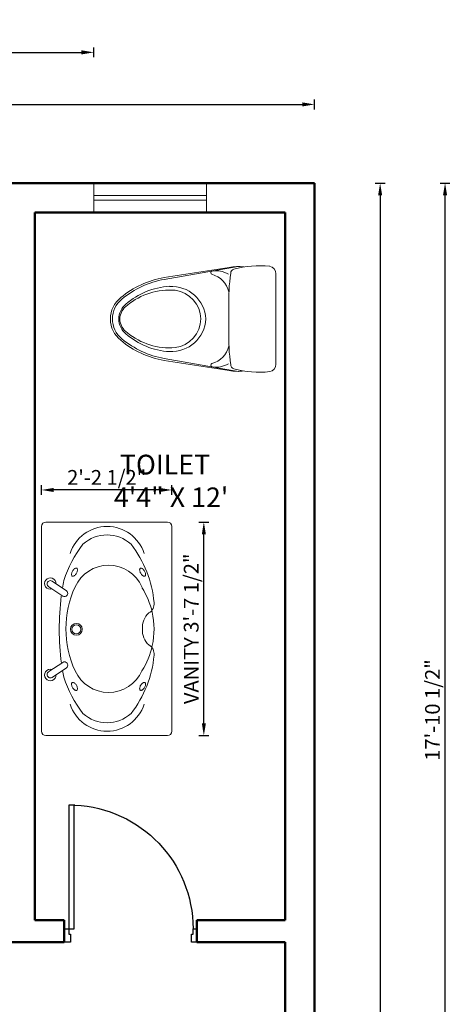
# Model space of a CAD drawing. Units: inches. Extents: x 1961 to 3038, y 800 to 1438.
# Tile 13 of 13: x 2949 to 3038, y 1148 to 1348. Entities that reach past the tile are written whole.
import ezdxf

# ---------------------------------------------------------------- set-up
doc = ezdxf.new("R2010")
doc.units = ezdxf.units.IN
for name, color, linetype, lineweight in [('A-ANNO-DIMS', 2, 'Continuous', 18), ('A-AREA-IDEN', 7, 'Continuous', 25), ('A-DOOR', 3, 'Continuous', 25), ('A-FLOR-FIXT', 9, 'Continuous', 18), ('A-GLAZ', 4, 'Continuous', 18), ('A-WALL', 7, 'Continuous', 50)]:
    doc.layers.add(name, color=color, linetype=linetype, lineweight=lineweight)
doc.styles.get("Standard").update_dxf_attribs({"font": 'arial.ttf'})
doc.dimstyles.new('ISO-25', dxfattribs={"dimtxt": 3, "dimasz": 2.5, "dimexe": 1, "dimexo": 1, "dimtad": 1, "dimdec": 4, "dimlunit": 4, "dimtxsty": 'Standard', "dimcen": 2.5, "dimadec": 0, "dimazin": 0, "dimtfac": 1, "dimtdec": 4, "dimtmove": 0, "dimatfit": 3, "dimfxl": 1, "dimfxlon": 1, "dimarcsym": 0})

# ---------------------------------------------------------------- blocks, each defined once
blk = doc.blocks.new('door 23')
for p, q in [((2995, 1217.93), (2996.24, 1217.93)), ((2995.15, 1192.78), (2995.15, 1217.93)), ((2996.24, 1217.93), (2996.24, 1192.78)), ((2997.17, 1192.78), (2995.15, 1192.78)), ((2996.24, 1192.78), (2996.24, 1191.69)), ((2996.24, 1191.69), (2995.91, 1191.69)), ((2995.91, 1191.69), (2995.91, 1190.05)), ((2995.91, 1190.05), (2997.17, 1190.05))]:
    blk.add_line(p, q)
blk.add_lwpolyline([(2970.17, 1190.05), (2971.26, 1190.05), (2971.26, 1191.69), (2970.93, 1191.69), (2970.93, 1192.78), (2970.17, 1192.78)])
blk.add_arc((2996.1, 1192.78), 25.17, 92.4896, 180)
blk = doc.blocks.new('A$C50C07CDD')
for p, q in [((1.8337, 1.1444), (0.039, 1.1444)), ((0, 1.1054), (0, 0.039)), ((0.511, 1.051), (0.5946, 0.9255)), ((0.5609, 1.0791), (0.6426, 0.9566)), ((1.304, 1.0791), (1.2223, 0.9566)), ((1.3539, 1.051), (1.2702, 0.9255)), ((1.8727, 0.039), (1.8727, 1.1054)), ((0.4107, 0.8636), (0.4061, 0.8593)), ((0.416, 0.8677), (0.4107, 0.8636)), ((0.4217, 0.8713), (0.416, 0.8677)), ((0.4278, 0.8745), (0.4217, 0.8713)), ((0.4339, 0.877), (0.4278, 0.8745)), ((0.44, 0.8789), (0.4339, 0.877)), ((0.4458, 0.88), (0.44, 0.8789)), ((0.4512, 0.8803), (0.4458, 0.88)), ((0.4559, 0.8798), (0.4512, 0.8803)), ((0.46, 0.8786), (0.4559, 0.8798)), ((0.4632, 0.8766), (0.46, 0.8786)), ((0.4654, 0.874), (0.4632, 0.8766)), ((0.4666, 0.8707), (0.4654, 0.874)), ((0.4657, 0.8629), (0.4667, 0.867)), ((0.4667, 0.867), (0.4666, 0.8707)), ((0.6281, 0.9168), (0.6347, 0.9201)), ((1.2368, 0.9168), (1.2302, 0.9201)), ((1.3982, 0.867), (1.3983, 0.8707)), ((1.3992, 0.8629), (1.3982, 0.867)), ((1.3983, 0.8707), (1.3995, 0.874)), ((1.3995, 0.874), (1.4017, 0.8766)), ((1.4017, 0.8766), (1.4049, 0.8786)), ((1.4049, 0.8786), (1.4089, 0.8798)), ((1.4089, 0.8798), (1.4137, 0.8803)), ((1.4137, 0.8803), (1.4191, 0.88)), ((1.4191, 0.88), (1.4249, 0.8789)), ((1.4249, 0.8789), (1.431, 0.877)), ((1.431, 0.877), (1.4371, 0.8745)), ((1.4371, 0.8745), (1.4432, 0.8713)), ((1.4432, 0.8713), (1.4489, 0.8677)), ((1.4489, 0.8677), (1.4542, 0.8636)), ((1.4542, 0.8636), (1.4588, 0.8593)), ((0.3973, 0.8459), (0.3963, 0.8418)), ((0.3963, 0.8418), (0.3964, 0.8381)), ((0.3964, 0.8381), (0.3976, 0.8349)), ((0.3993, 0.8503), (0.3973, 0.8459)), ((0.3976, 0.8349), (0.3998, 0.8322)), ((0.4022, 0.8548), (0.3993, 0.8503)), ((0.3998, 0.8322), (0.403, 0.8302)), ((0.4061, 0.8593), (0.4022, 0.8548)), ((0.403, 0.8302), (0.4071, 0.829)), ((0.4071, 0.829), (0.4118, 0.8286)), ((0.4118, 0.8286), (0.4172, 0.8289)), ((0.4172, 0.8289), (0.423, 0.83)), ((0.423, 0.83), (0.4291, 0.8318)), ((0.4291, 0.8318), (0.4352, 0.8343)), ((0.4352, 0.8343), (0.4413, 0.8375)), ((0.4413, 0.8375), (0.447, 0.8411)), ((0.447, 0.8411), (0.4523, 0.8452)), ((0.4523, 0.8452), (0.4569, 0.8495)), ((0.4569, 0.8495), (0.4608, 0.854)), ((0.4608, 0.854), (0.4637, 0.8585)), ((0.4637, 0.8585), (0.4657, 0.8629)), ((1.4012, 0.8585), (1.3992, 0.8629)), ((1.4041, 0.854), (1.4012, 0.8585)), ((1.408, 0.8495), (1.4041, 0.854)), ((1.4126, 0.8452), (1.408, 0.8495)), ((1.4179, 0.8411), (1.4126, 0.8452)), ((1.4236, 0.8375), (1.4179, 0.8411)), ((1.4296, 0.8343), (1.4236, 0.8375)), ((1.4358, 0.8318), (1.4296, 0.8343)), ((1.4419, 0.83), (1.4358, 0.8318)), ((1.4477, 0.8289), (1.4419, 0.83)), ((1.453, 0.8286), (1.4477, 0.8289)), ((1.4578, 0.829), (1.453, 0.8286)), ((1.4619, 0.8302), (1.4578, 0.829)), ((1.4588, 0.8593), (1.4626, 0.8548)), ((1.465, 0.8322), (1.4619, 0.8302)), ((1.4626, 0.8548), (1.4656, 0.8503)), ((1.4673, 0.8349), (1.465, 0.8322)), ((1.4656, 0.8503), (1.4676, 0.8459)), ((1.4684, 0.8381), (1.4673, 0.8349)), ((1.4676, 0.8459), (1.4686, 0.8418)), ((1.4686, 0.8418), (1.4684, 0.8381)), ((0.3963, 0.2691), (0.3964, 0.2729)), ((0.3973, 0.265), (0.3963, 0.2691)), ((0.3964, 0.2729), (0.3976, 0.2761)), ((0.3993, 0.2607), (0.3973, 0.265)), ((0.3976, 0.2761), (0.3998, 0.2788)), ((0.4022, 0.2562), (0.3993, 0.2607)), ((0.3998, 0.2788), (0.403, 0.2807)), ((0.403, 0.2807), (0.4071, 0.282)), ((0.4071, 0.282), (0.4118, 0.2824)), ((0.4118, 0.2824), (0.4172, 0.2821)), ((0.4172, 0.2821), (0.423, 0.281)), ((0.423, 0.281), (0.4291, 0.2792)), ((0.4291, 0.2792), (0.4352, 0.2766)), ((0.4352, 0.2766), (0.4413, 0.2735)), ((0.4413, 0.2735), (0.447, 0.2698)), ((0.447, 0.2698), (0.4523, 0.2658)), ((0.4523, 0.2658), (0.4569, 0.2614)), ((0.4569, 0.2614), (0.4608, 0.257)), ((1.408, 0.2614), (1.4041, 0.257)), ((1.4126, 0.2658), (1.408, 0.2614)), ((1.4179, 0.2698), (1.4126, 0.2658)), ((1.4236, 0.2735), (1.4179, 0.2698)), ((1.4296, 0.2766), (1.4236, 0.2735)), ((1.4358, 0.2792), (1.4296, 0.2766)), ((1.4419, 0.281), (1.4358, 0.2792)), ((1.4477, 0.2821), (1.4419, 0.281)), ((1.453, 0.2824), (1.4477, 0.2821)), ((1.4578, 0.282), (1.453, 0.2824)), ((1.4619, 0.2807), (1.4578, 0.282)), ((1.465, 0.2788), (1.4619, 0.2807)), ((1.4626, 0.2562), (1.4656, 0.2607)), ((1.4673, 0.2761), (1.465, 0.2788)), ((1.4656, 0.2607), (1.4676, 0.265)), ((1.4684, 0.2729), (1.4673, 0.2761)), ((1.4676, 0.265), (1.4686, 0.2691)), ((1.4686, 0.2691), (1.4684, 0.2729)), ((0.4061, 0.2517), (0.4022, 0.2562)), ((0.4107, 0.2473), (0.4061, 0.2517)), ((0.416, 0.2433), (0.4107, 0.2473)), ((0.4217, 0.2396), (0.416, 0.2433)), ((0.4278, 0.2365), (0.4217, 0.2396)), ((0.4339, 0.234), (0.4278, 0.2365)), ((0.44, 0.2321), (0.4339, 0.234)), ((0.4458, 0.231), (0.44, 0.2321)), ((0.4512, 0.2307), (0.4458, 0.231)), ((0.4559, 0.2312), (0.4512, 0.2307)), ((0.46, 0.2324), (0.4559, 0.2312)), ((0.4632, 0.2344), (0.46, 0.2324)), ((0.4608, 0.257), (0.4637, 0.2525)), ((0.4654, 0.237), (0.4632, 0.2344)), ((0.4637, 0.2525), (0.4657, 0.2481)), ((0.4666, 0.2402), (0.4654, 0.237)), ((0.4657, 0.2481), (0.4667, 0.244)), ((0.4667, 0.244), (0.4666, 0.2402)), ((1.3992, 0.2481), (1.3982, 0.244)), ((1.3982, 0.244), (1.3983, 0.2402)), ((1.3983, 0.2402), (1.3995, 0.237)), ((1.4012, 0.2525), (1.3992, 0.2481)), ((1.3995, 0.237), (1.4017, 0.2344)), ((1.4041, 0.257), (1.4012, 0.2525)), ((1.4017, 0.2344), (1.4049, 0.2324)), ((1.4049, 0.2324), (1.4089, 0.2312)), ((1.4089, 0.2312), (1.4137, 0.2307)), ((1.4137, 0.2307), (1.4191, 0.231)), ((1.4191, 0.231), (1.4249, 0.2321)), ((1.4249, 0.2321), (1.431, 0.234)), ((1.431, 0.234), (1.4371, 0.2365)), ((1.4371, 0.2365), (1.4432, 0.2396)), ((1.4432, 0.2396), (1.4489, 0.2433)), ((1.4489, 0.2433), (1.4542, 0.2473)), ((1.4542, 0.2473), (1.4588, 0.2517)), ((1.4588, 0.2517), (1.4626, 0.2562)), ((0.039, 0), (1.8337, 0))]:
    blk.add_line(p, q)
for radius in [0.052, 0.039]:
    blk.add_circle((0.9324, 0.8378), radius)
for centre, radius, start, end in [((0.039, 1.1054), 0.039, 90, 180), ((1.8337, 1.1054), 0.039, 0, 90), ((0.5314, 1.0667), 0.0499, 342.74842, 272.76223), ((0.5345, 1.0667), 0.0283, 25.16351, 213.6899), ((1.3335, 1.0667), 0.0499, 267.23783, 197.25158), ((1.3304, 1.0667), 0.0283, 326.31004, 154.83649), ((0.9363, -1.2974), 2.2857, 99.16732, 100.68241), ((0.9363, -1.2974), 2.2857, 82.769, 97.58301), ((0.6209, 0.9422), 0.026, 301.93729, 33.68995), ((1.244, 0.9422), 0.026, 146.31011, 238.06271), ((0.9363, -1.2974), 2.2857, 79.31759, 81.01168), ((0.3789, 0.568), 0.3407, 107.67047, 252.32953), ((0.8529, -0.0788), 1.0824, 108.31885, 127.47569), ((0.9363, 0.0502), 0.8799, 65.19892, 114.80107), ((0.6163, 0.9399), 0.026, 213.68988, 297.09225), ((1.2486, 0.9399), 0.026, 242.90775, 326.31012), ((1.0198, -0.0788), 1.0824, 52.52431, 71.68115), ((1.4938, 0.568), 0.3407, 287.67046, 72.32954), ((0.4262, 0.5699), 0.3131, 137.79286, 222.52497), ((0.7011, 0.5555), 0.3225, 114.51458, 245.48542), ((1.1716, 0.5555), 0.3225, 294.51459, 65.48541), ((1.4465, 0.5699), 0.3131, 317.47504, 42.20713), ((0.7926, 1.1239), 0.9718, 231.98414, 264.84793), ((1.0787, 1.1239), 0.9718, 275.15207, 308.01587), ((0.9324, 0.8378), 0.6817, 237.61175, 257.83778), ((0.9324, 0.8378), 0.6817, 282.71117, 302.38825), ((0.7165, 0.2459), 0.0906, 262.87503, 330.25511), ((0.9324, 0.8378), 0.6817, 257.83778, 282.71117), ((0.9199, 0.0927), 0.1652, 84.54609, 139.05674), ((0.9513, 0.0927), 0.1652, 40.94326, 95.45393), ((1.1547, 0.2459), 0.0906, 209.74489, 277.12497), ((0.039, 0.039), 0.039, 180, 270), ((1.8337, 0.039), 0.039, 270, 0)]:
    blk.add_arc(centre, radius, start, end)
blk = doc.blocks.new('A$C188A4A68')
at = {"ltscale": 20}
for p, q in [((0.2444, 0.7693), (0.0344, 0.7693)), ((0.2444, 0.7693), (0.4544, 0.7693)), ((0.0013, 0.5938), (0.0607, 0.2504)), ((0.0054, 0.5515), (0.0519, 0.2489)), ((0.2444, 0.5498), (0.1889, 0.5498)), ((0.2444, 0.5498), (0.2998, 0.5498)), ((0.4874, 0.5938), (0.428, 0.2504)), ((0.4833, 0.5515), (0.4368, 0.2489))]:
    blk.add_line(p, q, dxfattribs=at)
for centre, radius, start, end in [((0.442, 0.6914), 0.4447, 173.6395, 195.464), ((0.0344, 0.7343), 0.0349, 90, 169.5926), ((0.4544, 0.7343), 0.0349, 10.4074, 90), ((0.0467, 0.6914), 0.4447, 344.536, 6.3605), ((0.2125, 0.5932), 0.2113, 172.6498, 191.3659), ((0.2762, 0.5932), 0.2113, 348.6341, 7.3502), ((0.0333, 0.5802), 0.0213, 200.243, 267.1503), ((0.1303, 0.4913), 0.1097, 148.5069, 190.0488), ((0.1632, 1.4554), 0.906, 261.6902, 271.6258), ((0.1461, 0.4405), 0.1134, 104.1041, 164.1501), ((0.3255, 1.4554), 0.906, 268.3742, 278.3098), ((0.3426, 0.4405), 0.1134, 15.8499, 75.8959), ((0.3584, 0.4913), 0.1097, 349.9512, 31.4931), ((0.4554, 0.5802), 0.0213, 272.8497, 339.757), ((0.0297, 0.4734), 0.0075, 189.8264, 345.0875), ((0.459, 0.4734), 0.0075, 194.9125, 350.1736), ((0.254, 0.2824), 0.1613, 93.4333, 183.0038), ((0.2493, 0.2813), 0.1393, 92.0329, 172.0373), ((0.2347, 0.2824), 0.1613, 356.9962, 86.5667), ((0.2394, 0.2813), 0.1393, 7.9627, 87.9671), ((0.4211, 0.2752), 0.3108, 175.3213, 219.2477), ((0.0676, 0.2752), 0.3108, 320.7523, 4.6787), ((0.4781, 0.3243), 0.4328, 190.0297, 219.7428), ((0.4781, 0.3243), 0.4238, 190.0435, 219.7538), ((0.4311, 0.2946), 0.3389, 183.5042, 221.0229), ((0.0576, 0.2946), 0.3389, 318.9771, 356.4958), ((0.0106, 0.3243), 0.4238, 320.2462, 349.9565), ((0.0106, 0.3243), 0.4328, 320.2572, 349.9703), ((0.2444, 0.127), 0.127, 218.716, 270), ((0.2444, 0.127), 0.118, 218.6774, 270), ((0.2444, 0.127), 0.088, 218.504, 270), ((0.2498, 0.1282), 0.0854, 215.5685, 266.3197), ((0.2389, 0.1282), 0.0854, 273.6803, 324.4315), ((0.2444, 0.127), 0.088, 270, 321.496), ((0.2444, 0.127), 0.118, 270, 321.3226), ((0.2444, 0.127), 0.127, 270, 321.284)]:
    blk.add_arc(centre, radius, start, end, dxfattribs=at)
blk = doc.blocks.new('*D25')
at = {"layer": 'A-ANNO-DIMS', "color": 0, "lineweight": -2, "transparency": 16777216}
for p, q in [((2624.77, 1329.92), (2624.77, 1331.92)), ((2627.27, 1330.92), (3006.27, 1330.92)), ((3008.77, 1329.92), (3008.77, 1331.92))]:
    blk.add_line(p, q, dxfattribs=at)
at = {"layer": 'A-ANNO-DIMS', "color": 0, "transparency": 16777216}
for points in [[(2627.27, 1331.34), (2627.27, 1330.51), (2624.77, 1330.92)], [(3006.27, 1331.34), (3006.27, 1330.51), (3008.77, 1330.92)]]:
    blk.add_solid(points, dxfattribs=at)
at = {"layer": 'Defpoints', "color": 0, "transparency": 16777216}
for p in [(3008.77, 1330.92), (2624.77, 1314.92), (3008.77, 1314.92)]:
    blk.add_point(p, dxfattribs=at)
at = {"layer": 'A-ANNO-DIMS', "color": 0, "transparency": 16777216, "insert": (2816.77, 1333.08), "char_height": 3, "attachment_point": 5}
blk.add_mtext("32'", dxfattribs=at)
blk = doc.blocks.new('*D26')
at = {"layer": 'A-ANNO-DIMS', "color": 0, "lineweight": -2, "transparency": 16777216}
for p, q in [((3021.14, 1314.92), (3023.14, 1314.92)), ((3022.14, 1312.42), (3022.14, 855.42)), ((3021.14, 852.92), (3023.14, 852.92))]:
    blk.add_line(p, q, dxfattribs=at)
at = {"layer": 'A-ANNO-DIMS', "color": 0, "transparency": 16777216}
for points in [[(3021.72, 1312.42), (3022.55, 1312.42), (3022.14, 1314.92)], [(3021.72, 855.42), (3022.55, 855.42), (3022.14, 852.92)]]:
    blk.add_solid(points, dxfattribs=at)
at = {"layer": 'Defpoints', "color": 0, "transparency": 16777216}
for p in [(3008.77, 1314.92), (3008.77, 852.92), (3022.14, 852.92)]:
    blk.add_point(p, dxfattribs=at)
at = {"layer": 'A-ANNO-DIMS', "color": 0, "transparency": 16777216, "insert": (3019.98, 1083.92), "char_height": 3, "attachment_point": 5, "rotation": 90}
blk.add_mtext('38\'-6"', dxfattribs=at)
blk = doc.blocks.new('WIN-23IN')
for p, q in [((0, 23), (6, 23)), ((2.5, 23), (2.5, 0)), ((3.5, 23), (3.5, 0)), ((0, 0), (6, 0))]:
    blk.add_line(p, q)
blk = doc.blocks.new('*D65')
at = {"layer": 'A-ANNO-DIMS', "color": 0, "lineweight": -2, "transparency": 16777216}
for p, q in [((2985.21, 1245.93), (2987.21, 1245.93)), ((2986.21, 1204.95), (2986.21, 1243.43)), ((2985.21, 1202.45), (2987.21, 1202.45))]:
    blk.add_line(p, q, dxfattribs=at)
at = {"layer": 'A-ANNO-DIMS', "color": 0, "transparency": 16777216}
for points in [[(2985.8, 1243.43), (2986.63, 1243.43), (2986.21, 1245.93)], [(2985.8, 1204.95), (2986.63, 1204.95), (2986.21, 1202.45)]]:
    blk.add_solid(points, dxfattribs=at)
at = {"layer": 'Defpoints', "color": 0, "transparency": 16777216}
for p in [(2979.69, 1245.93), (2986.21, 1245.93), (2979.69, 1202.45)]:
    blk.add_point(p, dxfattribs=at)
at = {"layer": 'A-ANNO-DIMS', "color": 0, "transparency": 16777216, "insert": (2984.03, 1224.19), "char_height": 3, "attachment_point": 5, "rotation": 90}
blk.add_mtext('VANITY 3\'-7 1/2"', dxfattribs=at)
blk = doc.blocks.new('*D66')
at = {"layer": 'A-ANNO-DIMS', "color": 0, "lineweight": -2, "transparency": 16777216}
for p, q in [((2953.12, 1251.45), (2953.12, 1253.45)), ((2979.69, 1251.45), (2979.69, 1253.45)), ((2977.19, 1252.45), (2955.62, 1252.45))]:
    blk.add_line(p, q, dxfattribs=at)
at = {"layer": 'A-ANNO-DIMS', "color": 0, "transparency": 16777216}
for points in [[(2955.62, 1252.86), (2955.62, 1252.03), (2953.12, 1252.45)], [(2977.19, 1252.86), (2977.19, 1252.03), (2979.69, 1252.45)]]:
    blk.add_solid(points, dxfattribs=at)
at = {"layer": 'Defpoints', "color": 0, "transparency": 16777216}
for p in [(2953.12, 1252.45), (2953.12, 1245.93), (2979.69, 1245.93)]:
    blk.add_point(p, dxfattribs=at)
at = {"layer": 'A-ANNO-DIMS', "color": 0, "transparency": 16777216, "insert": (2966.41, 1254.62), "char_height": 3, "attachment_point": 5}
blk.add_mtext('2\'-2 1/2"', dxfattribs=at)
blk = doc.blocks.new('*D78')
at = {"layer": 'A-ANNO-DIMS', "color": 0, "lineweight": -2, "transparency": 16777216}
for p, q in [((2887.27, 1340.52), (2887.27, 1342.52)), ((2889.77, 1341.52), (2961.27, 1341.52)), ((2963.77, 1340.52), (2963.77, 1342.52))]:
    blk.add_line(p, q, dxfattribs=at)
at = {"layer": 'A-ANNO-DIMS', "color": 0, "transparency": 16777216}
for points in [[(2889.77, 1341.94), (2889.77, 1341.1), (2887.27, 1341.52)], [(2961.27, 1341.94), (2961.27, 1341.1), (2963.77, 1341.52)]]:
    blk.add_solid(points, dxfattribs=at)
at = {"layer": 'Defpoints', "color": 0, "transparency": 16777216}
for p in [(2963.77, 1341.52), (2887.27, 1314.92), (2963.77, 1314.92)]:
    blk.add_point(p, dxfattribs=at)
at = {"layer": 'A-ANNO-DIMS', "color": 0, "transparency": 16777216, "insert": (2925.52, 1343.7), "char_height": 3, "attachment_point": 5}
blk.add_mtext('6\'-4 1/2"', dxfattribs=at)
blk = doc.blocks.new('*D83')
at = {"layer": 'A-ANNO-DIMS', "color": 0, "lineweight": -2, "transparency": 16777216}
for p, q in [((3034.37, 1314.92), (3036.37, 1314.92)), ((3035.37, 1102.92), (3035.37, 1312.42)), ((3034.37, 1100.42), (3036.37, 1100.42))]:
    blk.add_line(p, q, dxfattribs=at)
at = {"layer": 'A-ANNO-DIMS', "color": 0, "transparency": 16777216}
for points in [[(3034.95, 1312.42), (3035.78, 1312.42), (3035.37, 1314.92)], [(3034.95, 1102.92), (3035.78, 1102.92), (3035.37, 1100.42)]]:
    blk.add_solid(points, dxfattribs=at)
at = {"layer": 'Defpoints', "color": 0, "transparency": 16777216}
for p in [(3008.77, 1314.92), (3035.37, 1314.92), (3008.77, 1100.42)]:
    blk.add_point(p, dxfattribs=at)
at = {"layer": 'A-ANNO-DIMS', "color": 0, "transparency": 16777216, "insert": (3033.19, 1207.67), "char_height": 3, "attachment_point": 5, "rotation": 90}
blk.add_mtext('17\'-10 1/2"', dxfattribs=at)

msp = doc.modelspace()

# ---------------------------------------------------------------- linework, layer by layer
at = {"layer": 'A-WALL'}
for p, q in [((3008.76803, 1314.91975), (2624.76803, 1314.91975)), ((3008.76803, 852.91975), (3008.76803, 1314.91975)), ((3002.76803, 1308.91975), (2951.76803, 1308.91975)), ((2951.76803, 1308.91975), (2951.76803, 1164.91975)), ((3002.76803, 1164.91975), (3002.76803, 1308.91975)), ((2957.76803, 1164.91975), (2951.76803, 1164.91975)), ((2957.76803, 1164.91975), (2957.76803, 1160.41975)), ((3002.76803, 1164.91975), (2984.76803, 1164.91975)), ((2984.76803, 1164.91975), (2984.76803, 1160.41975)), ((2957.76803, 1160.41975), (2842.26803, 1160.41975)), ((3002.76803, 1160.41975), (2984.76803, 1160.41975)), ((3002.76803, 975.41975), (3002.76803, 1160.41975))]:
    msp.add_line(p, q, dxfattribs=at)

# ---------------------------------------------------------------- block references
at = {"layer": 'A-DOOR', "xscale": -1}
msp.add_blockref('door 23', (5954.93509, -29.6271), dxfattribs=at)
at = {"layer": 'A-FLOR-FIXT'}
for name, p, xscale, yscale, zscale, rotation in [('A$C188A4A68', (2967.17807, 1297.97093), 43.8549224568521, 43.8549224568521, 43.8549224568521, 270), ('A$C50C07CDD', (2979.6903, 1202.44664), 23.21730682737528, 23.21730682737528, 23.21730682737528, 90)]:
    msp.add_blockref(name, p, dxfattribs=dict(at, xscale=xscale, yscale=yscale, zscale=zscale, rotation=rotation))
at = {"layer": 'A-GLAZ', "rotation": 90.00000000000479}
msp.add_blockref('WIN-23IN', (2986.76779, 1308.91972), dxfattribs=at)

# ---------------------------------------------------------------- texts
at = {"layer": 'A-AREA-IDEN', "insert": (2967.89061, 1259.62362), "char_height": 4, "attachment_point": 1}
msp.add_mtext_dynamic_manual_height_columns('{\\fTimes New Roman|b1|i0|c0|p18; TOILET\\P4\'4" X 12\'}', width=33.1080891, gutter_width=12.5, heights=[0], dxfattribs=at)

# ---------------------------------------------------------------- dimensions: what is measured, and where the dimension line sits
at = {"layer": 'A-ANNO-DIMS'}
for base, p1, p2, override, picture, middle in [((2963.76803, 1341.51975), (2887.26803, 1314.91975), (2963.76803, 1314.91975), {"dimdec": 1, "dimlfac": 1, "dimrnd": 0, "dimzin": 1, "dimdsep": 46, "dimlunit": 4, "dimfrac": 2}, '*D78', (2925.51803, 1343.69591)), ((3008.76803, 1330.92264), (2624.76803, 1314.91975), (3008.76803, 1314.91975), {"dimclrd": 0, "dimclre": 0, "dimclrt": 0}, '*D25', (2816.76803, 1333.08038))]:
    dim = msp.add_linear_dim(base=base, p1=p1, p2=p2, dimstyle='ISO-25', override=override, dxfattribs=at)
    dim.commit()
    dim.dimension.update_dxf_attribs({"geometry": picture, "text_midpoint": middle})
for base, p1, p2, angle, override, picture, middle in [((3022.1353, 852.91975), (3008.76803, 1314.91975), (3008.76803, 852.91975), 90, {"dimclrd": 0, "dimclre": 0, "dimclrt": 0}, '*D26', (3019.97756, 1083.91975)), ((3035.36803, 1314.91975), (3008.76803, 1100.41975), (3008.76803, 1314.91975), 90, {"dimdec": 1, "dimlfac": 1, "dimrnd": 0, "dimzin": 1, "dimdsep": 46, "dimlunit": 4, "dimfrac": 2}, '*D83', (3033.19187, 1207.66975)), ((2953.11989, 1252.44731), (2979.6903, 1245.92549), (2953.11989, 1245.92549), 180, {"dimdec": 1, "dimlfac": 1, "dimrnd": 0, "dimzin": 1, "dimdsep": 46, "dimlunit": 4, "dimfrac": 2}, '*D66', (2966.4051, 1254.62347))]:
    dim = msp.add_linear_dim(base=base, p1=p1, p2=p2, angle=angle, dimstyle='ISO-25', override=override, dxfattribs=at)
    dim.commit()
    dim.dimension.update_dxf_attribs({"geometry": picture, "text_midpoint": middle})
dim = msp.add_linear_dim(base=(2986.21213, 1245.92549), p1=(2979.6903, 1202.44664), p2=(2979.6903, 1245.92549), angle=90, text='VANITY <>', dimstyle='ISO-25', override={"dimdec": 1, "dimlfac": 1, "dimrnd": 0, "dimzin": 1, "dimdsep": 46, "dimlunit": 4, "dimfrac": 2}, dxfattribs=at)
dim.commit()
dim.dimension.update_dxf_attribs({"geometry": '*D65', "text_midpoint": (2984.03494, 1224.18606)})

doc.saveas('drawing.dxf')
